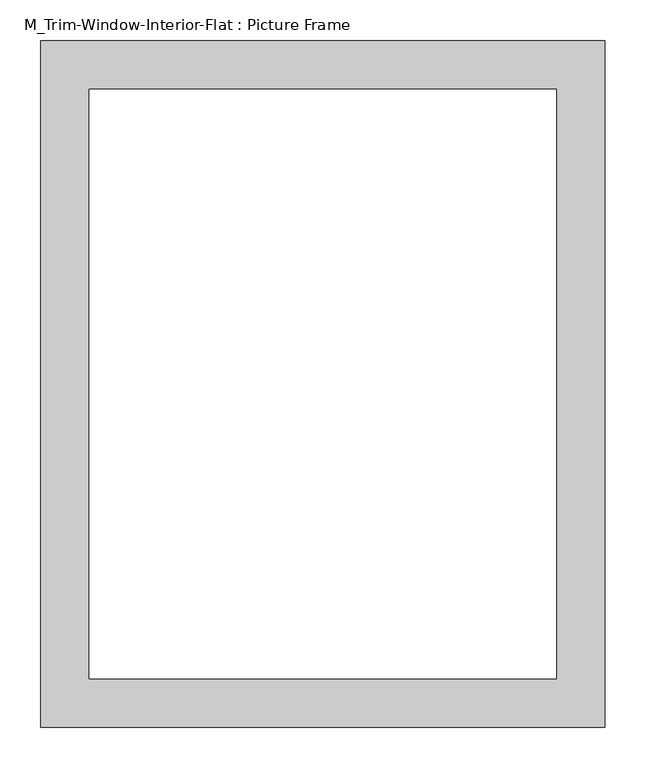
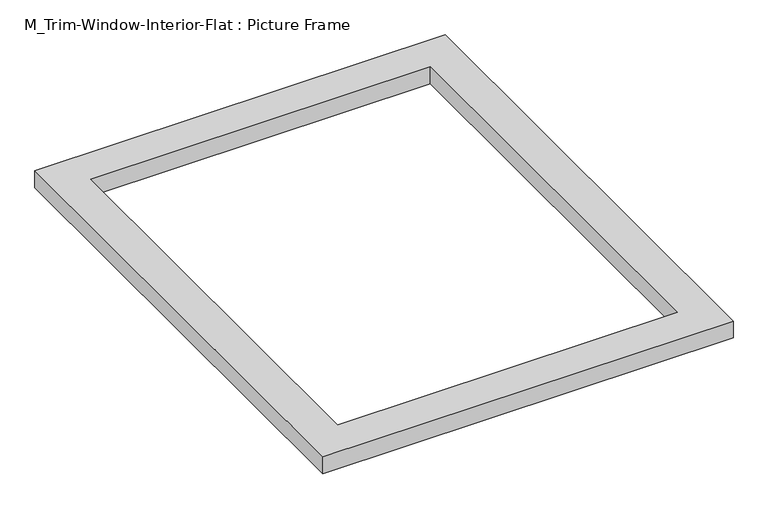
"""IFC4 building model written with IfcOpenShell, lengths in millimetres: proxy geometry, M_Trim-Window-Interior-Flat : Picture Frame."""

from ifc_helpers import new_model, si_unit, origin, origin_with_axes, place, context, project, spatial, polyline, outline, extrude, source, transform, mapped, element, save


def m_trim_window_interior_flat_picture_frame_c0d0133e(model_context):
    return source(origin(), model_context, "Body", "SweptSolid", [
        extrude(outline(polyline([(347.3, 47.3), (347.3, -797.3), (-347.3, -797.3), (-347.3, 47.3), (347.3, 47.3)]), holes=[polyline([(287.3, -12.7), (-287.3, -12.7), (-287.3, -737.3), (287.3, -737.3), (287.3, -12.7)])]), origin_with_axes(), (0.0, 0.0, 1.0), 30.0),
    ])


if __name__ == "__main__":
    model = new_model("IFC4")
    model_context = context("Model", 3, world=origin())
    ifc_project = project(units=[si_unit("LENGTHUNIT", "METRE", prefix="MILLI")], contexts=[model_context])
    site = spatial("IfcSite", under=ifc_project)
    building = spatial("IfcBuilding", under=site)
    placement = place(None, origin())
    m_trim_window_interior_flat_picture_frame_shape = m_trim_window_interior_flat_picture_frame_c0d0133e(model_context)
    element("IfcBuildingElementProxy", 1, Name="M_Trim-Window-Interior-Flat : Picture Frame", ObjectType="M_Trim-Window-Interior-Flat : Picture Frame", at=placement, inside=building, context=model_context, shape_type="MappedRepresentation", body=[
        mapped(m_trim_window_interior_flat_picture_frame_shape, transform((0.0, 0.0, 0.0), x_axis=(1.0, 0.0, 0.0), y_axis=(0.0, 1.0, 0.0), z_axis=(0.0, 0.0, 1.0))),
    ])
    save(model, "model.ifc")

# Revit data of these elements
# Type "M_Trim-Window-Interior-Flat : Picture Frame"
#   Trim Thickness_Picture Frame = 0.03 m
#   Trim Width = 0.06 m
#   Trim Thickness_with Sill = 0.02 m
#   Sill Thickness = 0.03 m
#   Opening Width [instance default] = 0.6 m
#   Opening Height [instance default] = 0.9 m
#   Default Elevation = 1.2 m
#   Sill = no
#   Picture Frame = yes
#   Trim Material [instance default] = none
# Element 1 (IfcBuildingElementProxy, "M_Trim-Window-Interior-Flat : Picture Frame")
#   Opening Height = 0.75 m
#   Trim Material = Wood - Stained
#   Materials on its faces: "Wood - Stained"
# Materials
#   "Wood - Stained": class "Wood", colour RGB 224 178 126, transparency 0, Cost = 0
